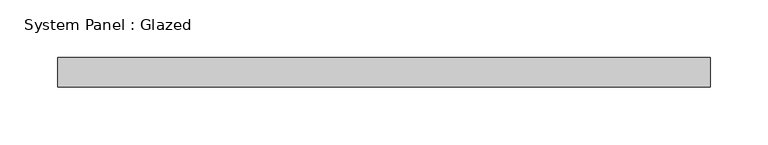
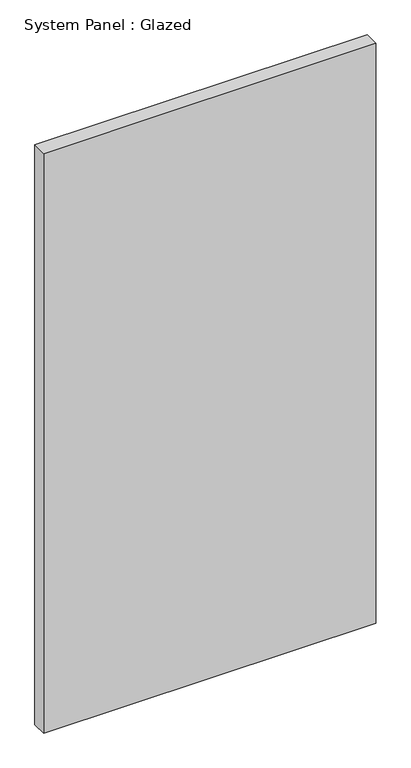
"""IFC4 building model written with IfcOpenShell, lengths in millimetres: plate geometry, System Panel : Glazed."""

from ifc_helpers import new_model, si_unit, origin, origin_with_axes, place, context, project, spatial, polyline, outline, extrude, source, transform, mapped, element, save


def system_panel_glazed_8b0ca3bf(model_context):
    return source(origin(), model_context, "Body", "SweptSolid", [
        extrude(outline(polyline([(282.575, 19.05), (-282.575, 19.05), (-282.575, 44.45), (282.575, 44.45), (282.575, 19.05)])), origin_with_axes(), (0.0, 0.0, 1.0), 1042.1148635),
    ])


if __name__ == "__main__":
    model = new_model("IFC4")
    model_context = context("Model", 3, world=origin())
    ifc_project = project(units=[si_unit("LENGTHUNIT", "METRE", prefix="MILLI")], contexts=[model_context])
    site = spatial("IfcSite", under=ifc_project)
    building = spatial("IfcBuilding", under=site)
    placement = place(None, origin())
    system_panel_glazed_shape = system_panel_glazed_8b0ca3bf(model_context)
    element("IfcPlate", 1, ObjectType="System Panel : Glazed", at=placement, inside=building, context=model_context, shape_type="MappedRepresentation", body=[
        mapped(system_panel_glazed_shape, transform((0.0, 0.0, 0.0), x_axis=(1.0, 0.0, 0.0), y_axis=(0.0, 1.0, 0.0), z_axis=(0.0, 0.0, 1.0))),
    ])
    save(model, "model.ifc")

# Revit data of these elements
# Type "System Panel : Glazed"
#   Construction Type Id = "GSP4R"
#   Analytic Construction = "1/8 in Pilkington single glazing"
#   Visual Light Transmittance = 0.9
#   Solar Heat Gain Coefficient = 0.86
#   Heat Transfer Coefficient (U) = 1.18115 BTU/(h·ft²·°F)
#   Define Thermal Properties by = 1
# Element 1 (IfcPlate, "System Panel : Glazed")
#   Materials on its faces: "Glass"
# Materials
#   "Glass": class "Glass", colour RGB 0 128 192, transparency 0.75, Description = "Soda Lime Glass", Cost = 0
